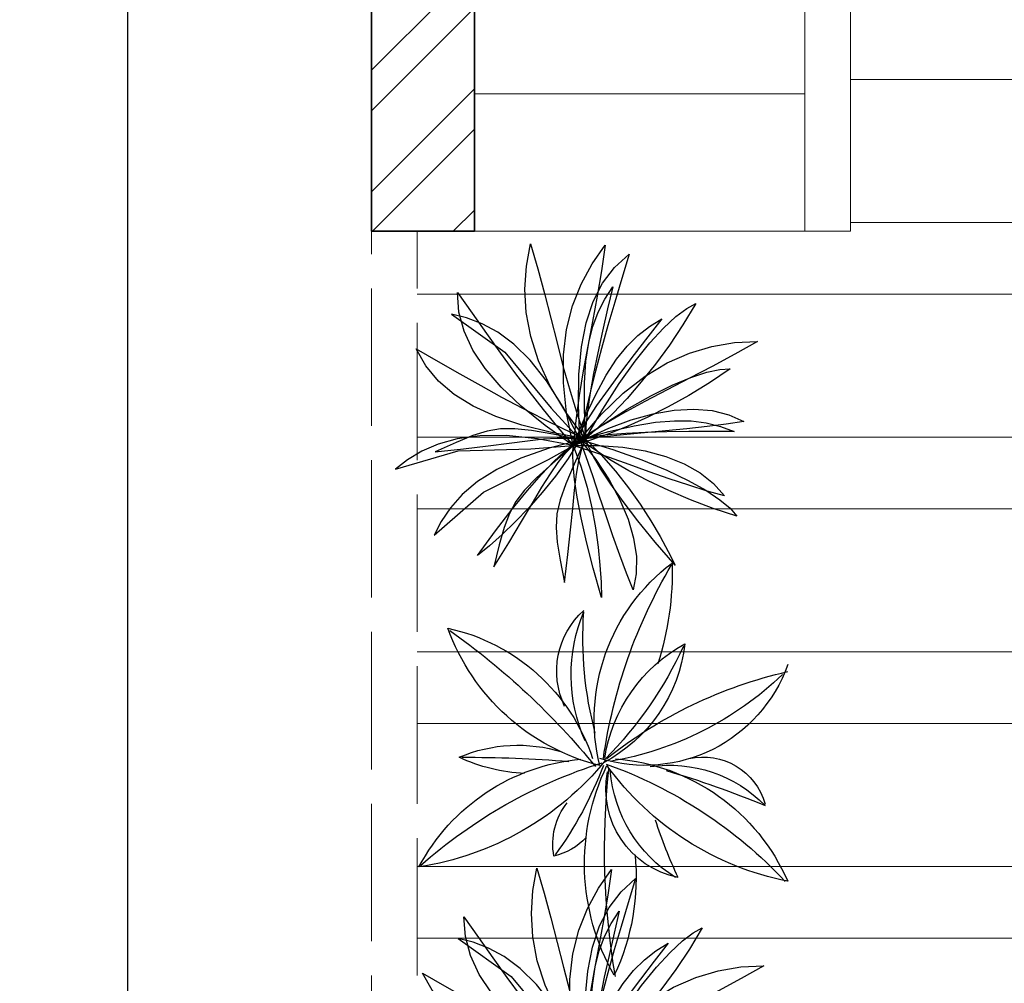
# Model space of a CAD drawing. Units: inches. Extents: x 351 to 1738, y -265 to 286.
# Tile 13 of 38: x 1004 to 1090, y -147 to -63. Entities that reach past the tile are written whole.
import ezdxf

# ---------------------------------------------------------------- set-up
doc = ezdxf.new("R2010")
doc.units = ezdxf.units.IN
doc.header["$MEASUREMENT"] = 0
doc.linetypes.add('ACAD_ISO02W100', pattern=[15, 12, -3])
for name, color, linetype, lineweight in [('A-ANNO-DIMS', 2, 'Continuous', 18), ('A-FLOR-OVHD', 1, 'ACAD_ISO02W100', 18), ('A-FLOR-PATT', 9, 'Continuous', 9), ('A-FLOR-STRS', 7, 'Continuous', 18), ('A-WALL', 7, 'Continuous', 35), ('A-WALL-PATT', 152, 'Continuous', 13)]:
    doc.layers.add(name, color=color, linetype=linetype, lineweight=lineweight)
for name, color, linetype in [('CAY', 94, 'Continuous'), ('CHITIET', 144, 'Continuous'), ('DIENHOA', 3, 'Continuous'), ('netmanh', 9, 'Continuous'), ('VATDUNG', 9, 'Continuous')]:
    doc.layers.add(name, color=color, linetype=linetype)
doc.styles.get("Standard").update_dxf_attribs({"font": 'arial.ttf'})
doc.dimstyles.get("Standard").update_dxf_attribs({"dimtxt": 8, "dimasz": 5, "dimexe": 0.18, "dimexo": 0.0625, "dimgap": 0.09, "dimtad": 1, "dimtoh": 1, "dimzin": 0, "dimdsep": 46, "dimlunit": 4, "dimtxsty": 'Standard', "dimcen": 0, "dimclre": 256, "dimadec": 0, "dimazin": 0, "dimtfac": 1, "dimtofl": 0, "dimtmove": 0, "dimatfit": 3, "dimfxl": 1, "dimtolj": 1, "dimtzin": 0, "dimlwe": -1, "dimarcsym": 0})

# ---------------------------------------------------------------- blocks, each defined once
blk = doc.blocks.new('*D8')
at = {"layer": 'A-ANNO-DIMS', "color": 0, "transparency": 16777216}
for p, q in [((1034.642, 255.963), (1013.221, 255.963)), ((1034.642, -203.037), (1013.221, -203.037))]:
    blk.add_line(p, q, dxfattribs=at)
at = {"layer": 'A-ANNO-DIMS', "color": 0, "lineweight": -2, "transparency": 16777216}
blk.add_line((1013.401, 250.963), (1013.401, -198.037), dxfattribs=at)
at = {"layer": 'A-ANNO-DIMS', "color": 0, "transparency": 16777216}
for points in [[(1012.568, 250.963), (1014.235, 250.963), (1013.401, 255.963)], [(1012.568, -198.037), (1014.235, -198.037), (1013.401, -203.037)]]:
    blk.add_solid(points, dxfattribs=at)
at = {"layer": 'Defpoints', "color": 0, "transparency": 16777216}
for p in [(1034.704, 255.963), (1013.401, -203.037), (1034.704, -203.037)]:
    blk.add_point(p, dxfattribs=at)
at = {"layer": 'A-ANNO-DIMS', "color": 0, "transparency": 16777216, "insert": (1009.224, 26.463), "char_height": 8, "attachment_point": 5, "rotation": 90}
blk.add_mtext('\\A1;38\'-3"', dxfattribs=at)
blk = doc.blocks.new('A$C5431134F')
at = {"layer": 'VATDUNG'}
for centre, radius, start, end in [((2160.8, 1662), 1245, 150.2411, 205.809), ((5177, 1582.5), 4150.3, 170.24, 186.1148), ((-65.9, 1738.8), 1267.2, 354.3326, 25.2804), ((193.1, 3473.3), 2507.8, 289.6318, 316.9416), ((2357.8, 162.2), 1629.1, 101.2486, 143.9899), ((1000.7, 2213.1), 1133.8, 274.4073, 336.4431), ((1532.8, 1250.1), 499, 101.4267, 190.9877), ((1828.1, 1082.8), 773.2, 121.9055, 175.1859), ((3715.1, 660.2), 2523.5, 154.6853, 162.4501), ((-246.7, 51.1), 1647.5, 39.15, 81.389), ((1000.7, 2213.1), 1133.8, 208.0484, 264.6491), ((1859.5, 3770.4), 2797.6, 228.5745, 252.3842), ((1101.5, 1552.5), 361.2, 169.1166, 218.9556), ((667.9, 1279.8), 349.9, 42.8374, 76.9786), ((-929.9, 388.9), 2082.1, 20.5138, 36.0242), ((1386.4, 1856.4), 738.5, 261.6389, 315.6255), ((-169.9, 6392.7), 5465.7, 286.3355, 292.415), ((1571.2, 1428.8), 356.3, 257.3557, 344.3532), ((624.5, 223.6), 940.4, 92.4374, 115.2956), ((1294.4, -49.6), 1206.1, 104.1284, 160.1468), ((-2233.8, 3749.8), 4146.2, 305.4464, 320.7382), ((248.9, 8461.8), 7388, 269.91003, 274.50199), ((2052.7, 864.5), 1083.3, 166.3603, 232.9474), ((1250.8, 281.5), 836.9, 19.4342, 107.4357), ((625, 349.3), 851.8, 6.5073, 62.3609), ((-65.9, 1738.8), 1267.2, 330.7697, 331.9367), ((754.1, -691.9), 1814.1, 46.1483, 80.3711), ((-70, 1420), 1084.7, 282.2423, 341.7321), ((546.4, 1826.6), 819.5, 246.7315, 287.3971), ((3885.3, 1488.7), 2894, 188.0959, 210.7226), ((1889.6, 1210.8), 871.9, 188.5552, 241.3289), ((-527.8, -458.7), 2192.5, 24.7599, 44.6473), ((2594.9, 3037.7), 2500, 231.5416, 257.1764), ((1738.9, 617.5), 897.6, 155.9893, 202.84), ((2946.5, 414), 2039.9, 165.0604, 184.0737), ((1214.1, 597.8), 452.1, 154.5276, 228.0163), ((-246.7, 51.1), 1647.5, 358.2222, 17.8583)]:
    blk.add_arc(centre, radius, start, end, dxfattribs=at)
blk = doc.blocks.new('A$C5A8625A6')
at = {"layer": 'CHITIET', "ltscale": 50, "xscale": -0.49, "yscale": 0.49, "zscale": 0.49, "rotation": 180}
blk.add_blockref('A$C5431134F', (0, 1120.2), dxfattribs=at)
blk = doc.blocks.new('A$C18571848')
at = {"layer": 'netmanh', "xscale": 0.5393606399999998, "yscale": 0.5393606399999998, "zscale": 0.5393606399999998}
blk.add_blockref('A$C5A8625A6', (0, 0), dxfattribs=at)
blk = doc.blocks.new('Cay03_mb')
at = {"layer": 'DIENHOA'}
for p, q in [((118.6, 555.3), (166.2, 599.1)), ((166.2, 599.1), (142.2, 519.4)), ((79.5, 503.7), (118.6, 555.3)), ((142.2, 519.4), (119, 441.7)), ((48.6, 443.6), (79.5, 503.7)), ((25.5, 374.3), (48.6, 443.6)), ((119, 441.7), (96.7, 365.6)), ((-365.2, 390.3), (-414.4, 402.8)), ((-414.4, 402.8), (-240.2, 277.8)), ((-314.9, 371.3), (-365.2, 390.3)), ((-263.5, 343.5), (-314.9, 371.3)), ((9.9, 295.3), (25.5, 374.3)), ((96.7, 365.6), (75.6, 290.6)), ((-211.2, 304.6), (-263.5, 343.5)), ((-158, 252.3), (-211.2, 304.6)), ((1.6, 205.7), (9.9, 295.3)), ((75.6, 290.6), (55.7, 216.3)), ((363.4, 275.4), (436.8, 297.2)), ((436.8, 297.2), (511, 309.6)), ((511, 309.6), (585.9, 313.5)), ((585.9, 313.5), (511.8, 271.4)), ((-240.2, 277.8), (-88.4, 94.9)), ((290.6, 243.2), (363.4, 275.4)), ((511.8, 271.4), (437.6, 231.5)), ((-104.2, 184.4), (-158, 252.3)), ((218.5, 199.8), (290.6, 243.2)), ((437.6, 231.5), (363.7, 192.9)), ((0.2, 104.9), (1.6, 205.7)), ((55.7, 216.3), (37.3, 142.1)), ((147, 144.1), (218.5, 199.8)), ((-49.6, 98.5), (-104.2, 184.4)), ((363.7, 192.9), (290.2, 154.9)), ((37.3, 142.1), (20.5, 67.6)), ((75.9, 75.2), (147, 144.1)), ((290.2, 154.9), (217.4, 116.6)), ((5.4, -7.8), (-49.6, 98.5)), ((5.4, -7.8), (0.2, 104.9)), ((217.4, 116.6), (145.5, 77.3)), ((-88.4, 94.9), (5.4, -7.8)), ((5.4, -7.8), (75.9, 75.2)), ((20.5, 67.6), (5.4, -7.8)), ((145.5, 77.3), (74.7, 36.1)), ((74.7, 36.1), (5.4, -7.8)), ((100.3, 18.4), (182.2, 37.2)), ((182.2, 37.2), (253, 48.9)), ((253, 48.9), (314.6, 54.1)), ((314.6, 54.1), (369.2, 53.3)), ((369.2, 53.3), (418.6, 46.8)), ((418.6, 46.8), (464.9, 35.2)), ((464.9, 35.2), (510, 19)), ((-345, 5.4), (-399.6, -17.1)), ((-298.6, 20.1), (-345, 5.4)), ((-254.7, 27.4), (-298.6, 20.1)), ((-208, 27.8), (-254.7, 27.4)), ((-152.7, 21.7), (-208, 27.8)), ((-83.4, 9.7), (-152.7, 21.7)), ((5.4, -7.8), (-83.4, 9.7)), ((5.4, -7.8), (100.3, 18.4)), ((46.3, 0.9), (5.4, -7.8)), ((96.7, 7.5), (46.3, 0.9)), ((155, 12.2), (96.7, 7.5)), ((219.6, 15.4), (155, 12.2)), ((289, 17.4), (219.6, 15.4)), ((361.6, 18.5), (289, 17.4)), ((435.8, 18.9), (361.6, 18.5)), ((510, 19), (435.8, 18.9)), ((-399.6, -17.1), (-468, -47.9)), ((-375.6, -37.8), (-295.3, -27.9)), ((-295.3, -27.9), (-225.8, -18.9)), ((-225.8, -18.9), (-165.8, -11.3)), ((-165.8, -11.3), (-114, -5.7)), ((-114, -5.7), (-69, -2.9)), ((-69, -2.9), (-29.6, -3.4)), ((-45.1, -46.3), (-16.5, -22.4)), ((5.4, -7.8), (-33.2, -69.5)), ((-29.6, -3.4), (5.4, -7.8)), ((-16.5, -22.4), (5.4, -7.8)), ((5.4, -7.8), (56.8, -73.3)), ((25.9, -64.4), (5.4, -7.8)), ((5.4, -7.8), (112.8, -40.3)), ((53.5, -41.6), (5.4, -7.8)), ((-468, -47.9), (-375.6, -37.8)), ((-79.8, -79.6), (-45.1, -46.3)), ((47, -125.9), (25.9, -64.4)), ((107, -75.7), (53.5, -41.6)), ((112.8, -40.3), (207.5, -73.8)), ((-120.2, -122.1), (-79.8, -79.6)), ((-33.2, -69.5), (-74.6, -127.3)), ((56.8, -73.3), (100.4, -139.1)), ((165.5, -109.6), (107, -75.7)), ((207.5, -73.8), (289.5, -107.6)), ((-165.9, -174.1), (-120.2, -122.1)), ((-74.6, -127.3), (-117.8, -181.1)), ((68.7, -190.6), (47, -125.9)), ((228.7, -142.8), (165.5, -109.6)), ((289.5, -107.6), (359.3, -141.1)), ((100.4, -139.1), (135.9, -204.3)), ((296, -174.7), (228.7, -142.8)), ((359.3, -141.1), (416.9, -173.5)), ((-216.3, -235.6), (-165.9, -174.1)), ((-117.8, -181.1), (-162.1, -230.9)), ((90.8, -256.6), (68.7, -190.6)), ((367.1, -204.8), (296, -174.7)), ((416.9, -173.5), (462.6, -204.2)), ((135.9, -204.3), (162.8, -268.3)), ((441.6, -232.7), (367.1, -204.8)), ((462.6, -204.2), (496.5, -232.5)), ((-271, -306.6), (-216.3, -235.6)), ((-162.1, -230.9), (-206.3, -276.5)), ((113.1, -322.2), (90.8, -256.6)), ((518.9, -257.7), (441.6, -232.7)), ((496.5, -232.5), (518.9, -257.7)), ((-206.3, -276.5), (-249.6, -317.8)), ((162.8, -268.3), (181, -330.4)), ((-329.5, -387.1), (-271, -306.6)), ((-249.6, -317.8), (-291, -354.7)), ((135.4, -385.6), (113.1, -322.2)), ((181, -330.4), (190, -390)), ((-291, -354.7), (-329.5, -387.1)), ((157.6, -445), (135.4, -385.6)), ((190, -390), (189.6, -446.3)), ((179.5, -498.7), (157.6, -445)), ((189.6, -446.3), (179.5, -498.7))]:
    blk.add_line(p, q, dxfattribs=at)
for points in [[(23.7, -5.4), (-41, 82.2), (-91.8, 167.1), (-129.7, 249.5), (-155.6, 329.6), (-170.2, 407.8), (-174.7, 484.2), (-169.8, 559.3), (-156.5, 633.1)], [(-156.5, 633.1), (-132.5, 551.3), (-110.5, 470), (-89.8, 389.2), (-69.6, 309), (-49, 229.4), (-27.1, 150.4), (-3.2, 72.1), (23.7, -5.4)], [(-16.4, -26.7), (-38.3, 80), (-48.9, 178.3), (-48.7, 269), (-38.5, 352.6), (-19.1, 429.7), (9, 501), (44.9, 567.1), (87.9, 628.5)], [(87.9, 628.5), (75.5, 544.2), (61.3, 461.2), (46.1, 379.1), (30.8, 297.8), (16.1, 216.9), (2.9, 136), (-8.3, 54.9), (-16.4, -26.7)], [(23.7, -5.4), (19.8, 93), (20.3, 177), (25, 248.5), (34, 309.8), (47.3, 362.7), (64.9, 409.3), (86.8, 451.7), (112.9, 491.9)], [(112.9, 491.9), (96, 419.7), (79.5, 347.4), (63.9, 276.5), (50, 208.4), (38.4, 144.8), (29.7, 86.9), (24.6, 36.3), (23.7, -5.4)], [(-395.6, 473.7), (-347.5, 405.6), (-300.6, 339.5), (-254.3, 275.1), (-208.3, 212.3), (-161.9, 150.9), (-114.8, 90.7), (-66.5, 31.6), (-16.4, -26.7)], [(-16.4, -26.7), (-108.3, 38.6), (-186.9, 101.7), (-252.4, 163.5), (-305.1, 224.4), (-345.4, 285.2), (-373.7, 346.6), (-390.4, 409.2), (-395.6, 473.7)], [(384.3, 437.5), (342.2, 367.8), (298.1, 301.7), (252.6, 239.4), (206.1, 181.1), (159.4, 127.2), (113, 78), (67.6, 33.6), (23.7, -5.4)], [(23.7, -5.4), (79.9, 91.7), (134.1, 176.2), (185.8, 248.4), (234.3, 308.7), (279, 357.3), (319.3, 394.8), (354.6, 421.4), (384.3, 437.5)], [(273.2, 387.3), (227.6, 328.8), (182.3, 270.1), (138.4, 212.3), (97.2, 156.4), (60, 103.4), (27.8, 54.6), (1.9, 10.8), (-16.4, -26.7)], [(-16.4, -26.7), (21.4, 64.2), (57, 140.3), (91.4, 203.3), (125.2, 255.1), (159.5, 297.5), (195, 332.5), (232.7, 361.8), (273.2, 387.3)], [(-530.5, 289.7), (-458.3, 248.1), (-387.9, 207.8), (-318.9, 168.7), (-250.8, 131.1), (-182.9, 94.8), (-114.9, 59.9), (-46.2, 26.5), (23.7, -5.4)], [(23.7, -5.4), (-87.2, 15.2), (-185, 39.6), (-270.3, 68.2), (-343.7, 101.4), (-405.9, 139.7), (-457.3, 183.5), (-498.7, 233.4), (-530.5, 289.7)], [(496.7, 224), (429.4, 178.4), (361.6, 136.9), (294.1, 99.5), (227.5, 66.1), (162.4, 36.7), (99.7, 11.5), (39.8, -9.7), (-16.4, -26.7)], [(-16.4, -26.7), (75.4, 37.9), (160.1, 91.8), (237.3, 135.7), (306.6, 170), (367.6, 195.4), (419.9, 212.5), (463.1, 221.9), (496.7, 224)], [(23.7, -5.4), (99.3, 29.7), (173.2, 57.1), (244.8, 76.7), (313.3, 88.3), (377.9, 91.8), (437.9, 87), (492.7, 73.8), (541.4, 52)], [(541.4, 52), (484.1, 42.9), (421.2, 34.8), (354.4, 27.6), (285.4, 20.9), (216.1, 14.5), (148.2, 8.1), (83.5, 1.6), (23.7, -5.4)], [(-16.4, -26.7), (-134, -4.7), (-235.3, 5.3), (-322, 4.7), (-395.9, -5), (-458.7, -22.3), (-512.3, -45.7), (-558.2, -73.6), (-598.4, -104.7)], [(-598.4, -104.7), (-392.7, -44.4), (-155, -37.4), (-16.4, -26.7)], [(-471.9, -320.3), (-310.5, -179.3), (-97.7, -73.3), (23.7, -5.4)], [(23.7, -5.4), (-92.3, -34.8), (-188.4, -68.2), (-266.9, -105.1), (-329.9, -144.9), (-379.7, -187), (-418.5, -230.7), (-448.5, -275.3), (-471.9, -320.3)], [(-276.2, -424.4), (-227.3, -345.4), (-185.7, -276.1), (-150, -215.7), (-119.1, -163.8), (-91.5, -119.5), (-66, -82.3), (-41.4, -51.6), (-16.4, -26.7)], [(-16.4, -26.7), (-84.9, -86), (-137, -133.1), (-175.8, -173), (-204.3, -210), (-225.5, -249.1), (-242.5, -294.7), (-258.4, -351.6), (-276.2, -424.4)], [(23.7, -5.4), (-13.6, -87.9), (-41.1, -152.6), (-59.6, -205), (-69.9, -250.7), (-72.8, -295), (-69.2, -343.6), (-59.7, -401.9), (-45.3, -475.5)], [(-45.3, -475.5), (-34.1, -383.2), (-25.4, -302.8), (-18.3, -233.1), (-12, -172.9), (-5.6, -121.2), (2, -76.8), (11.4, -38.5), (23.7, -5.4)], [(76.2, -524.2), (48.8, -428.5), (26.6, -341.7), (9.2, -264.1), (-3.6, -196.1), (-12.3, -138), (-17.1, -90.2), (-18.3, -53), (-16.4, -26.7)], [(-16.4, -26.7), (66.9, -26.6), (145.6, -32.7), (218.8, -44.9), (285.8, -63.1), (345.9, -87.1), (398.4, -116.6), (442.6, -151.6), (477.6, -191.8)], [(477.6, -191.8), (421.8, -176), (361.3, -156.9), (297.6, -135.5), (232.2, -112.6), (166.6, -89.4), (102.3, -66.6), (40.8, -45.4), (-16.4, -26.7)], [(-16.4, -26.7), (8.5, -95.1), (28.5, -163.3), (44.3, -230.6), (56.3, -296.1), (65, -359), (70.9, -418.5), (74.5, -473.9), (76.2, -524.2)], [(316.5, -418.1), (251.4, -342.8), (194.8, -273.3), (146.5, -210.2), (106.3, -153.8), (74.1, -104.7), (49.7, -63.4), (32.9, -30.1), (23.7, -5.4)], [(23.7, -5.4), (74.9, -57.1), (121.8, -110.6), (164.3, -165), (202.7, -219.4), (237, -272.9), (267.3, -324.5), (293.7, -373.2), (316.5, -418.1)]]:
    blk.add_lwpolyline(points, dxfattribs=at)

msp = doc.modelspace()

# ---------------------------------------------------------------- hatches: boundary and pattern name
at = {"layer": 'A-FLOR-PATT', "transparency": 33554559}
h = msp.add_hatch(dxfattribs=at)
h.set_pattern_fill('ANSI32', color=256, scale=50, angle=135)
h.set_pattern_definition([(180, (1038.704, -199.037), (-2e-15, -18.75), []), (180, (1032.454, -192.787), (-2e-15, -18.75), [])])
h.paths.add_polyline_path([(1248.506, -102.915), (1236.559, -102.916), (1236.553, -56.864), (1112.704, -57.026), (1112.704, -57.037), (1103.704, -57.037), (1103.704, -45.037), (1103.704, 98.963), (1076.434, 98.963), (1076.549, -81.037), (1071.549, -81.037), (1043.704, -81.037), (1038.704, -81.037), (1038.704, -161.037), (1043.704, -161.037), (1043.704, -173.037), (1038.704, -173.037), (1038.704, -199.037), (1562.704, -199.037), (1562.704, -173.037), (1236.549, -173.037), (1236.549, -164.037), (1236.693, -164.037), (1236.676, -150.916), (1248.512, -150.915)])
h.paths.add_polyline_path([(1236.133, -134.078), (1247.348, -134.078), (1247.348, -122.929), (1236.133, -122.929)], flags=24)
h.paths.add_polyline_path([(1308.144, -185.548), (1321.66, -185.548), (1321.66, -174.4), (1308.144, -174.4)], flags=24)
h.paths.add_polyline_path([(1121.632, -122.88), (1179.647, -122.88), (1179.647, -112.309), (1121.632, -112.309)], flags=24)
h.paths.add_polyline_path([(1124.515, -112.593), (1177.986, -112.593), (1177.986, -101.056), (1124.515, -101.056)], flags=24)
h.paths.add_polyline_path([(1091.374, 23.58), (1104.89, 23.58), (1104.89, 34.728), (1091.374, 34.728)], flags=24)
at = {"layer": 'A-WALL-PATT'}
h = msp.add_hatch(dxfattribs=at)
h.set_pattern_fill('ANSI32', color=256, scale=20)
h.set_pattern_definition([(45, (1034.704, -173.037), (-5.3033, 5.3033), []), (45, (1038.24, -173.037), (-5.3033, 5.3033), [])])
h.paths.add_polyline_path([(1043.704, -57.037), (1034.704, -57.037), (1034.704, -81.037), (1043.704, -81.037)])
h.paths.add_polyline_path([(1043.704, 198.963), (1034.704, 198.963), (1034.704, -45.037), (1043.704, -45.037)])
h.paths.add_polyline_path([(1043.704, 243.963), (1034.704, 243.963), (1034.704, 237.963), (1034.704, 210.963), (1043.704, 210.963)])
h.paths.add_polyline_path([(1112.704, 255.963), (1043.704, 255.963), (1043.704, 246.963), (1103.704, 246.963), (1103.704, 237.963), (1112.704, 237.963), (1112.704, 251.963)])
h.paths.add_polyline_path([(1056.704, 207.963), (1043.704, 207.963), (1043.704, 198.963), (1056.704, 198.963)])
h.paths.add_polyline_path([(1103.704, 207.963), (1092.704, 207.963), (1092.704, 198.963), (1103.704, 198.963)])
h.paths.add_polyline_path([(1112.704, 228.963), (1103.704, 228.963), (1103.704, 74.963), (1112.704, 74.963), (1112.704, 97.5)])
h.paths.add_polyline_path([(1284.129, -164.037), (1248.549, -164.037), (1248.549, -173.037), (1284.129, -173.037)])
h.paths.add_polyline_path([(1524.064, -164.037), (1472.204, -164.037), (1472.204, -138.5), (1468.204, -138.5), (1468.204, -164.037), (1344.129, -164.037), (1344.129, -173.037), (1524.064, -173.037)])
h.paths.add_polyline_path([(1384.204, -57.037), (1380.065, -57.037), (1380.204, -164.037), (1384.204, -164.037)])
h.paths.add_polyline_path([(1566.704, -138), (1557.704, -138), (1557.704, -164.037), (1536.064, -164.037), (1536.064, -173.037), (1566.704, -173.037)])
h.paths.add_polyline_path([(1566.704, -30.189), (1557.704, -30.189), (1557.704, -53.037), (1536.064, -53.037), (1536.064, -57.037), (1557.704, -57.037), (1557.704, -102), (1566.704, -102)])
h.paths.add_polyline_path([(1524.064, -53.037), (1442.549, -53.037), (1442.549, -57.037), (1468.204, -57.037), (1468.204, -102.5), (1472.204, -102.5), (1472.204, -57.037), (1524.064, -57.037)])
h.paths.add_polyline_path([(1566.704, 120.993), (1557.704, 120.993), (1557.704, 29.811), (1566.704, 29.811)])
h.paths.add_polyline_path([(1384.204, 64.463), (1380.204, 64.463), (1380.204, -3.5), (1384.204, -3.5)])
h.paths.add_polyline_path([(1266.549, 237.963), (1248.704, 237.963), (1248.704, 228.963), (1266.549, 228.963)])
h.paths.add_polyline_path([(1329.549, 237.963), (1302.549, 237.963), (1302.549, 228.963), (1329.549, 228.963)])
h.paths.add_polyline_path([(1380.204, 237.963), (1365.549, 237.963), (1365.549, 228.963), (1380.204, 228.963)])
h.paths.add_polyline_path([(1524.064, 237.963), (1392.204, 237.963), (1392.204, 228.963), (1524.064, 228.963)])
h.paths.add_polyline_path([(1384.204, 228.963), (1380.204, 228.963), (1380.204, 73.463), (1384.204, 73.463)])
h.paths.add_polyline_path([(1566.704, 237.963), (1536.064, 237.963), (1536.064, 228.963), (1557.704, 228.963), (1557.704, 180.993), (1566.704, 180.993)])

# ---------------------------------------------------------------- linework, layer by layer
at = {"layer": 'A-FLOR-OVHD'}
for p, q in [((1034.704, -203.037), (1034.704, -81.037)), ((1038.704, -161.037), (1038.704, -81.037))]:
    msp.add_line(p, q, dxfattribs=at)
at = {"layer": 'A-FLOR-STRS'}
for p, q in [((1072.549, -81.037), (1072.549, 162.963)), ((1076.394, 162.963), (1076.549, -81.037)), ((1043.704, -69.037), (1072.549, -69.037)), ((1043.704, -81.037), (1072.549, -81.037)), ((1076.549, -81.037), (1071.549, -81.037))]:
    msp.add_line(p, q, dxfattribs=at)
at = {"layer": 'A-WALL'}
for p, q in [((1034.704, 255.963), (1034.704, -81.037)), ((1043.704, 198.963), (1043.704, -81.037)), ((1034.704, -81.037), (1043.704, -81.037))]:
    msp.add_line(p, q, dxfattribs=at)

# ---------------------------------------------------------------- block references
at = {"layer": 'CAY'}
for name, p, xscale, yscale, zscale in [('Cay03_mb', (1052.772, -99.026), 0.0267074520028285, 0.0267074520028285, 0.0267074520028285), ('A$C18571848', (1038.852, -146.124), 0.0597507335965459, 0.0597507335965459, 0.0597507335965459), ('Cay03_mb', (1053.334, -153.565), 0.0267074520028285, 0.0267074520028285, 0.0267074520028285)]:
    msp.add_blockref(name, p, dxfattribs=dict(at, xscale=xscale, yscale=yscale, zscale=zscale))

# ---------------------------------------------------------------- dimensions: what is measured, and where the dimension line sits
at = {"layer": 'A-ANNO-DIMS'}
dim = msp.add_linear_dim(base=(1013.401, -203.037), p1=(1034.704, 255.963), p2=(1034.704, -203.037), angle=90, dimstyle='Standard', override={"dimclrd": 0, "dimclre": 0, "dimclrt": 0}, dxfattribs=at)
dim.commit()
dim.dimension.update_dxf_attribs({"geometry": '*D8', "text_midpoint": (1013.401, 26.463), "dimtype": 160})

doc.saveas('drawing.dxf')
